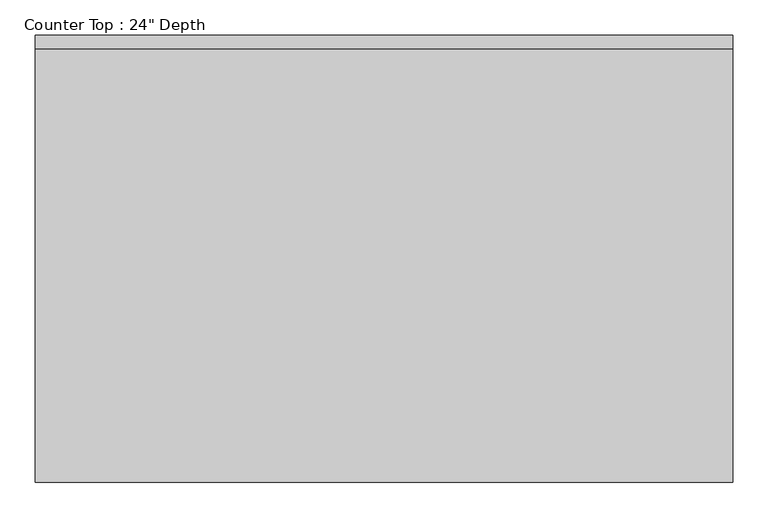
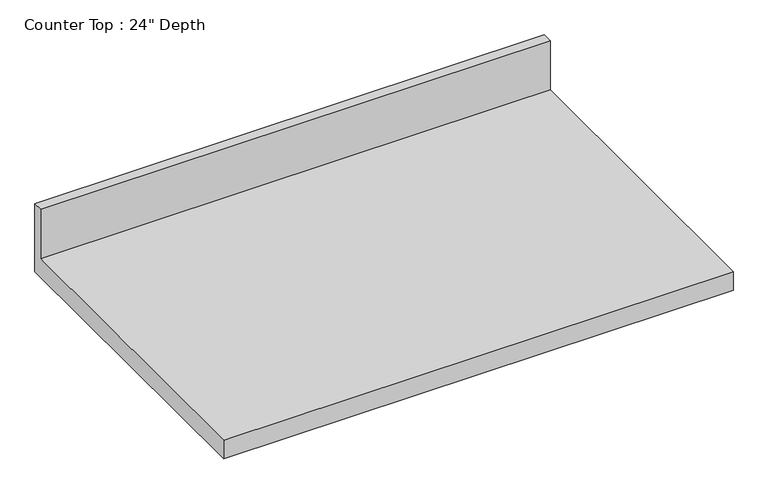
"""IFC4 building model written with IfcOpenShell, lengths in millimetres: furniture geometry."""

from ifc_helpers import new_model, si_unit, frame, origin, place, context, project, spatial, polyline, outline, extrude, source, transform, mapped, element, save


def furniture_47cc8d9a(model_context):
    return source(origin(), model_context, "Body", "SweptSolid", [
        extrude(outline(polyline([(0.0, 1016.0), (0.0, 876.3), (-635.0, 876.3), (-635.0, 914.4), (-19.05, 914.4), (-19.05, 1016.0), (0.0, 1016.0)])), frame((-1200.4622951, 0.0, 0.0), z_axis=(1.0, 0.0, 0.0), x_axis=(0.0, 1.0, 0.0)), (0.0, 0.0, 1.0), 990.6),
    ])


if __name__ == "__main__":
    model = new_model("IFC4")
    model_context = context("Model", 3, world=origin())
    ifc_project = project(units=[si_unit("LENGTHUNIT", "METRE", prefix="MILLI")], contexts=[model_context])
    site = spatial("IfcSite", under=ifc_project)
    building = spatial("IfcBuilding", under=site)
    placement = place(None, origin())
    furniture_shape = furniture_47cc8d9a(model_context)
    element("IfcFurniture", 1, ObjectType="Counter Top : 24\" Depth", at=placement, inside=building, context=model_context, shape_type="MappedRepresentation", body=[
        mapped(furniture_shape, transform((0.0, 0.0, 0.0), x_axis=(1.0, 0.0, 0.0), y_axis=(0.0, 1.0, 0.0), z_axis=(0.0, 0.0, 1.0))),
    ])
    save(model, "model.ifc")

# Revit data of these elements
# Type "Counter Top : 24\" Depth"
#   Assembly Code = "C1030400"
#   Counter Thickness = 0' - 1 1/2"
#   Depth = 2' - 1"
#   Height = 3' - 0"
#   Length [instance default] = 8' - 0"
#   Counter Top Material = none
#   Default Elevation = 0
# Element 1 (IfcFurniture, "Counter Top : 24\" Depth")
#   Length = 3' - 3"
#   Materials on its faces: "Counter Top"
# Materials
#   "Counter Top": class "Wood", colour RGB 226 177 128, transparency 0
